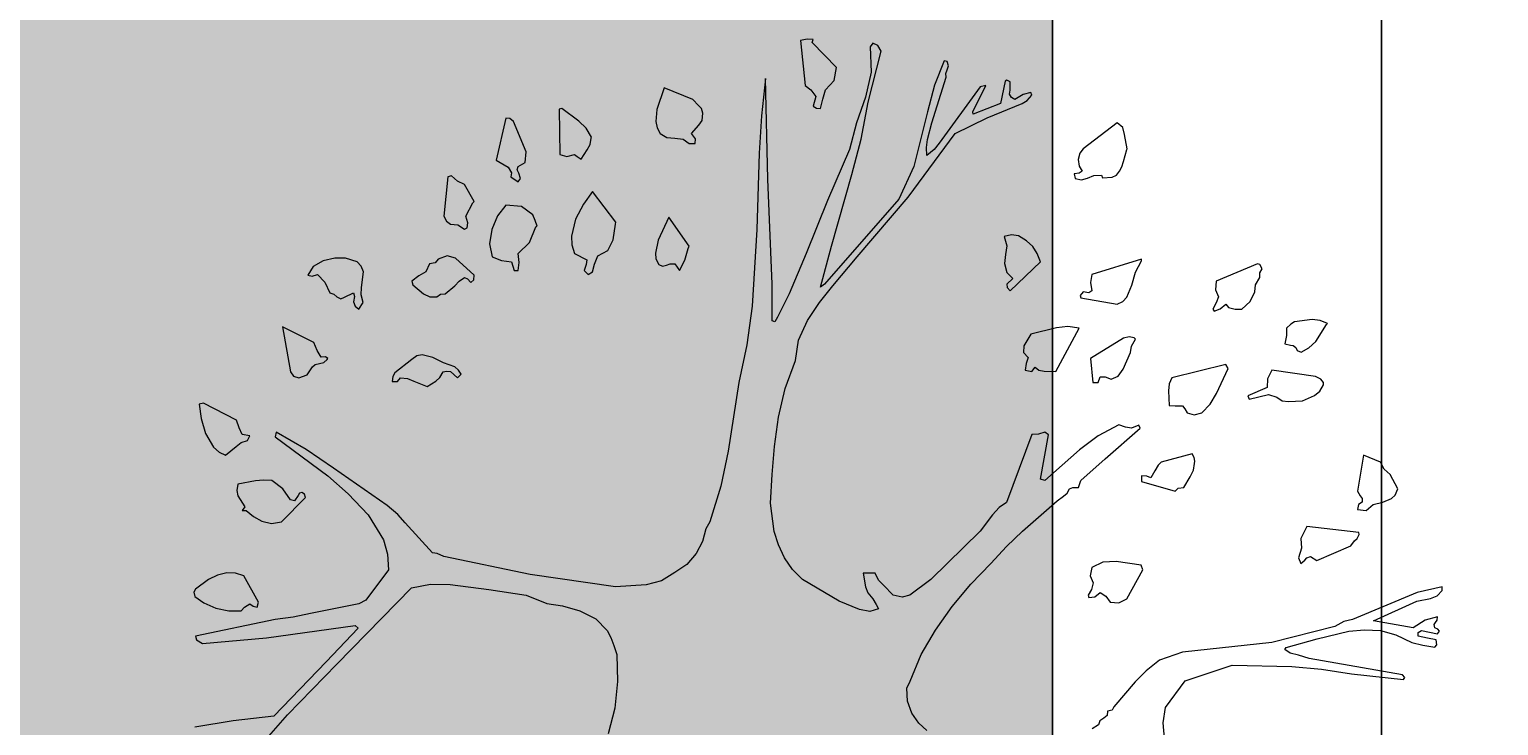
# Model space of a CAD drawing. Units: inches. Extents: x 84 to 1044, y -280 to 906.
# Tile 44 of 105: x 955 to 995, y -107 to -88. Entities that reach past the tile are written whole.
import ezdxf

# ---------------------------------------------------------------- set-up
doc = ezdxf.new("R2010")
doc.units = ezdxf.units.IN
for name, color, linetype, lineweight in [('A-ANNO-DIMS', 2, 'Continuous', 18), ('C-PROP', 7, 'Continuous', 25), ('L-PLNT', 114, 'Continuous', 15)]:
    doc.layers.add(name, color=color, linetype=linetype, lineweight=lineweight)
doc.layers.add('L-PLNT-PATT', color=9, linetype='Continuous', lineweight=9, true_color=0xafd9aa)
doc.styles.get("Standard").update_dxf_attribs({"font": 'arial.ttf'})
doc.dimstyles.get("Standard").update_dxf_attribs({"dimtxt": 0.18, "dimasz": 0.18, "dimexe": 0.18, "dimexo": 0.0625, "dimgap": 0.09, "dimtad": 0, "dimtih": 1, "dimtoh": 1, "dimdec": 4, "dimzin": 0, "dimdsep": 46, "dimtxsty": 'Standard', "dimcen": 0.09, "dimadec": 0, "dimazin": 0, "dimtfac": 1, "dimtdec": 4, "dimtofl": 0, "dimtmove": 0, "dimatfit": 3, "dimfxl": 1, "dimtolj": 1, "dimtzin": 0, "dimarcsym": 0})

# ---------------------------------------------------------------- blocks, each defined once
blk = doc.blocks.new('A$C37E508DF')
for p, q in [((0.6329, 1.5111), (0.6367, 1.5175)), ((0.6367, 1.5175), (0.6423, 1.5201)), ((0.6423, 1.5201), (0.6453, 1.5158)), ((0.6826, 1.493), (0.7096, 1.5209)), ((0.7083, 1.5239), (0.7152, 1.5244)), ((0.7096, 1.5209), (0.7083, 1.5239)), ((0.7152, 1.5244), (0.7225, 1.5231)), ((0.7225, 1.5231), (0.7174, 1.4729)), ((0.5596, 1.4995), (0.563, 1.5003)), ((0.563, 1.5003), (0.5737, 1.4733)), ((0.6475, 1.4545), (0.6329, 1.5111)), ((0.6453, 1.5158), (0.644, 1.4879)), ((0.5583, 1.4948), (0.5596, 1.4995)), ((0.5596, 1.4905), (0.5583, 1.4948)), ((0.5613, 1.4862), (0.5596, 1.4905)), ((0.5608, 1.4823), (0.5613, 1.4862)), ((0.644, 1.4879), (0.6505, 1.46)), ((0.6852, 1.4785), (0.6826, 1.493)), ((0.4897, 1.4772), (0.4935, 1.4789)), ((0.4897, 1.4678), (0.4897, 1.4772)), ((0.4905, 1.4635), (0.4897, 1.4678)), ((0.4935, 1.4789), (0.4952, 1.478)), ((0.4952, 1.478), (0.5004, 1.4532)), ((0.5313, 1.4437), (0.5167, 1.4729)), ((0.5167, 1.4729), (0.5231, 1.4716)), ((0.5231, 1.4716), (0.5686, 1.409)), ((0.5767, 1.4317), (0.5608, 1.4823)), ((0.5737, 1.4733), (0.5814, 1.4437)), ((0.6946, 1.4682), (0.6852, 1.4785)), ((0.6976, 1.4579), (0.6946, 1.4682)), ((0.7109, 1.4682), (0.7053, 1.4609)), ((0.7174, 1.4729), (0.7109, 1.4682)), ((0.7589, 1.3691), (0.7615, 1.481)), ((0.7615, 1.481), (0.7658, 1.4395)), ((0.8421, 1.4575), (0.8739, 1.4703)), ((0.8739, 1.4703), (0.882, 1.4463)), ((0.4657, 1.4622), (0.4669, 1.4652)), ((0.4708, 1.4566), (0.4657, 1.4622)), ((0.4669, 1.4652), (0.4755, 1.463)), ((0.4764, 1.4532), (0.4708, 1.4566)), ((0.4755, 1.463), (0.4845, 1.4575)), ((0.5154, 1.4373), (0.4764, 1.4532)), ((0.4845, 1.4575), (0.4884, 1.4596)), ((0.4884, 1.4596), (0.4905, 1.4635)), ((0.5004, 1.4532), (0.5308, 1.4412)), ((0.6552, 1.4137), (0.6475, 1.4545)), ((0.6505, 1.46), (0.6603, 1.4317)), ((0.7002, 1.4476), (0.6976, 1.4579)), ((0.7053, 1.4609), (0.7083, 1.4502)), ((0.8357, 1.451), (0.8421, 1.4575)), ((0.551, 1.4197), (0.5154, 1.4373)), ((0.5308, 1.4412), (0.5313, 1.4437)), ((0.5814, 1.4437), (0.5969, 1.3833)), ((0.7049, 1.448), (0.7002, 1.4476)), ((0.7083, 1.4502), (0.7049, 1.448)), ((0.7658, 1.4395), (0.7684, 1.3979)), ((0.831, 1.4424), (0.8323, 1.4476)), ((0.8318, 1.4343), (0.831, 1.4424)), ((0.8323, 1.4476), (0.8357, 1.451)), ((0.882, 1.4463), (0.8829, 1.433)), ((0.9686, 1.4334), (0.9875, 1.4476)), ((0.9875, 1.4476), (0.9905, 1.4467)), ((0.9905, 1.4467), (0.9896, 1.3966)), ((1.0411, 1.433), (1.045, 1.4365)), ((1.045, 1.4365), (1.0497, 1.4369)), ((1.0497, 1.4369), (1.0604, 1.3901)), ((0.3598, 1.403), (0.3628, 1.4189)), ((0.3628, 1.4189), (0.3649, 1.4266)), ((0.3649, 1.4266), (0.3709, 1.4317)), ((0.3709, 1.4317), (0.4086, 1.403)), ((0.6029, 1.3494), (0.551, 1.4197)), ((0.5814, 1.4133), (0.5767, 1.4317)), ((0.6603, 1.4317), (0.668, 1.4021)), ((0.8353, 1.4292), (0.8318, 1.4343)), ((0.8434, 1.4197), (0.8353, 1.4292)), ((0.8391, 1.4141), (0.8434, 1.4197)), ((0.8781, 1.4197), (0.8709, 1.4154)), ((0.8816, 1.4262), (0.8781, 1.4197)), ((0.8829, 1.433), (0.8816, 1.4262)), ((0.9545, 1.4159), (0.9605, 1.4257)), ((0.9605, 1.4257), (0.9686, 1.4334)), ((1.0269, 1.3996), (1.0411, 1.433)), ((0.3602, 1.4021), (0.3598, 1.403)), ((0.4086, 1.403), (0.4125, 1.3979)), ((0.5686, 1.409), (0.5741, 1.4021)), ((0.5827, 1.4043), (0.5814, 1.4133)), ((0.5823, 1.3953), (0.5827, 1.4043)), ((0.6655, 1.3743), (0.6552, 1.4137)), ((0.8395, 1.4086), (0.8391, 1.4141)), ((0.846, 1.4086), (0.8395, 1.4086)), ((0.8528, 1.4137), (0.846, 1.4086)), ((0.8619, 1.4146), (0.8528, 1.4137)), ((0.8709, 1.4154), (0.8619, 1.4146)), ((0.9549, 1.4146), (0.9545, 1.4159)), ((0.9558, 1.4077), (0.9549, 1.4146)), ((0.9592, 1.4017), (0.9558, 1.4077)), ((0.364, 1.3888), (0.3602, 1.4021)), ((0.3657, 1.3828), (0.364, 1.3888)), ((0.4125, 1.3979), (0.4142, 1.391)), ((0.4142, 1.391), (0.4134, 1.3837)), ((0.5741, 1.4021), (0.5823, 1.3953)), ((0.668, 1.4021), (0.6925, 1.3455)), ((0.7684, 1.3979), (0.771, 1.3134)), ((0.966, 1.3914), (0.9592, 1.4017)), ((0.9703, 1.3944), (0.966, 1.3914)), ((0.9733, 1.3966), (0.9703, 1.3944)), ((0.9819, 1.3944), (0.9733, 1.3966)), ((0.9896, 1.3966), (0.9819, 1.3944)), ((1.0282, 1.3876), (1.0269, 1.3996)), ((1.0359, 1.3833), (1.0282, 1.3876)), ((1.0604, 1.3901), (1.0471, 1.3824)), ((0.3683, 1.3781), (0.3657, 1.3828)), ((0.3718, 1.3738), (0.3683, 1.3781)), ((0.3765, 1.3713), (0.3718, 1.3738)), ((0.3872, 1.3708), (0.3765, 1.3713)), ((0.3885, 1.3738), (0.3872, 1.3708)), ((0.3971, 1.3734), (0.3885, 1.3738)), ((0.4039, 1.3704), (0.3971, 1.3734)), ((0.4108, 1.3683), (0.4039, 1.3704)), ((0.4134, 1.3837), (0.4099, 1.3781)), ((0.4099, 1.3781), (0.4134, 1.376)), ((0.4176, 1.37), (0.4108, 1.3683)), ((0.4134, 1.376), (0.4189, 1.3751)), ((0.4189, 1.3751), (0.4176, 1.37)), ((0.5969, 1.3833), (0.6132, 1.3472)), ((0.6882, 1.2949), (0.6655, 1.3743)), ((1.0334, 1.37), (1.0351, 1.376)), ((1.0359, 1.3661), (1.0334, 1.37)), ((1.0351, 1.376), (1.0368, 1.3794)), ((1.0368, 1.3794), (1.0359, 1.3833)), ((1.0441, 1.3717), (1.0359, 1.3661)), ((1.0471, 1.3824), (1.0432, 1.3764)), ((1.0432, 1.3764), (1.0441, 1.3717)), ((1.1033, 1.367), (1.1097, 1.373)), ((1.1097, 1.373), (1.114, 1.3717)), ((1.114, 1.3717), (1.1183, 1.328)), ((0.7538, 1.2529), (0.7589, 1.3691)), ((0.9274, 1.3215), (0.9532, 1.3554)), ((0.9532, 1.3554), (0.9635, 1.3413)), ((1.0848, 1.3443), (1.0955, 1.3631)), ((1.0955, 1.3631), (1.1033, 1.367)), ((0.6595, 1.2829), (0.6029, 1.3494)), ((0.6132, 1.3472), (0.6959, 1.2529)), ((0.6925, 1.3455), (0.7161, 1.2868)), ((0.9635, 1.3413), (0.9721, 1.325)), ((1.0197, 1.3297), (1.0321, 1.3387)), ((1.0321, 1.3387), (1.0497, 1.3404)), ((1.0497, 1.3404), (1.0587, 1.3284)), ((1.0861, 1.343), (1.0848, 1.3443)), ((1.0938, 1.328), (1.0861, 1.343)), ((0.846, 1.2949), (0.8687, 1.3271)), ((0.8687, 1.3271), (0.8803, 1.3014)), ((0.9279, 1.3194), (0.9274, 1.3215)), ((0.9721, 1.325), (0.9768, 1.3061)), ((1.0149, 1.3172), (1.0171, 1.3232)), ((1.0171, 1.3232), (1.0197, 1.3297)), ((1.0587, 1.3284), (1.0651, 1.3134)), ((1.0917, 1.3207), (1.0938, 1.328)), ((1.1153, 1.3228), (1.111, 1.3194)), ((1.1183, 1.328), (1.1153, 1.3228)), ((0.4717, 1.3009), (0.4807, 1.3065)), ((0.4807, 1.3065), (0.4884, 1.3074)), ((0.4884, 1.3074), (0.4965, 1.3057)), ((0.4965, 1.3057), (0.4935, 1.2954)), ((0.771, 1.3134), (0.7761, 1.2285)), ((0.9305, 1.3018), (0.9279, 1.3194)), ((0.9768, 1.3061), (0.9763, 1.2962)), ((1.0162, 1.3164), (1.0149, 1.3172)), ((1.0231, 1.2988), (1.0162, 1.3164)), ((1.0651, 1.3134), (1.0677, 1.2975)), ((1.0925, 1.3151), (1.0917, 1.3207)), ((1.0955, 1.3138), (1.0925, 1.3151)), ((1.1028, 1.3185), (1.0955, 1.3138)), ((1.111, 1.3194), (1.1028, 1.3185)), ((0.4597, 1.2868), (0.4648, 1.2945)), ((0.4648, 1.2945), (0.4717, 1.3009)), ((0.4935, 1.2954), (0.4948, 1.2855)), ((0.7002, 1.2495), (0.6882, 1.2949)), ((0.8473, 1.2924), (0.846, 1.2949)), ((0.8507, 1.2795), (0.8473, 1.2924)), ((0.8803, 1.3014), (0.8833, 1.2872)), ((0.9365, 1.2902), (0.9305, 1.3018)), ((0.9476, 1.2842), (0.9365, 1.2902)), ((0.9763, 1.2962), (0.9733, 1.2868)), ((1.0359, 1.2868), (1.0231, 1.2988)), ((1.0677, 1.2975), (1.0647, 1.2829)), ((0.2101, 1.2696), (0.2127, 1.2744)), ((0.2127, 1.2744), (0.2152, 1.2752)), ((0.2152, 1.2752), (0.2611, 1.2559)), ((0.3439, 1.2804), (0.3992, 1.2636)), ((0.3439, 1.2787), (0.3439, 1.2804)), ((0.3507, 1.2662), (0.3439, 1.2787)), ((0.4562, 1.2774), (0.4597, 1.2868)), ((0.4897, 1.2452), (0.4562, 1.2774)), ((0.4961, 1.2756), (0.4935, 1.2658)), ((0.4948, 1.2855), (0.4961, 1.2756)), ((0.6865, 1.2508), (0.6595, 1.2829)), ((0.7161, 1.2868), (0.7349, 1.2422)), ((0.8567, 1.2679), (0.8507, 1.2795)), ((0.8619, 1.2752), (0.8567, 1.2679)), ((0.867, 1.2752), (0.8619, 1.2752)), ((0.8713, 1.2739), (0.867, 1.2752)), ((0.8756, 1.2726), (0.8713, 1.2739)), ((0.8799, 1.2744), (0.8756, 1.2726)), ((0.8829, 1.2808), (0.8799, 1.2744)), ((0.8833, 1.2872), (0.8829, 1.2808)), ((0.951, 1.2748), (0.9476, 1.2842)), ((0.9532, 1.2666), (0.951, 1.2748)), ((0.9733, 1.2868), (0.9596, 1.2799)), ((0.9596, 1.2799), (0.9605, 1.2744)), ((0.9605, 1.2744), (0.9626, 1.2679)), ((1.0347, 1.2769), (1.0359, 1.2868)), ((1.0359, 1.2679), (1.0347, 1.2769)), ((1.0432, 1.2774), (1.0402, 1.2679)), ((1.0544, 1.2791), (1.0432, 1.2774)), ((1.0647, 1.2829), (1.0544, 1.2791)), ((1.0848, 1.2628), (1.1054, 1.2817)), ((1.1054, 1.2817), (1.1148, 1.2842)), ((1.1148, 1.2842), (1.1247, 1.2804)), ((1.1247, 1.2804), (1.1281, 1.2765)), ((1.1281, 1.2765), (1.1341, 1.2752)), ((1.1341, 1.2752), (1.1384, 1.2666)), ((1.2075, 1.2666), (1.21, 1.2726)), ((1.21, 1.2726), (1.2147, 1.2774)), ((1.2147, 1.2774), (1.2276, 1.2817)), ((1.2276, 1.2817), (1.2392, 1.2817)), ((1.2392, 1.2817), (1.2521, 1.2787)), ((1.2521, 1.2787), (1.2632, 1.2722)), ((1.2632, 1.2722), (1.2692, 1.2628)), ((0.2127, 1.2654), (0.2101, 1.2696)), ((0.2127, 1.2602), (0.2127, 1.2654)), ((0.2174, 1.2521), (0.2127, 1.2602)), ((0.2611, 1.2559), (0.262, 1.2465)), ((0.3546, 1.2516), (0.3507, 1.2662)), ((0.3992, 1.2636), (0.4005, 1.2546)), ((0.4935, 1.2658), (0.4867, 1.2589)), ((0.4867, 1.2589), (0.4935, 1.2529)), ((0.9583, 1.2636), (0.9532, 1.2666)), ((0.9626, 1.2679), (0.9583, 1.2636)), ((1.0402, 1.2679), (1.0359, 1.2679)), ((1.0852, 1.2576), (1.0848, 1.2628)), ((1.0883, 1.2546), (1.0852, 1.2576)), ((1.0921, 1.2585), (1.0883, 1.2546)), ((1.0955, 1.2602), (1.0921, 1.2585)), ((1.1015, 1.2559), (1.0955, 1.2602)), ((1.1063, 1.2508), (1.1015, 1.2559)), ((1.1384, 1.2666), (1.1461, 1.2619)), ((1.1461, 1.2619), (1.1539, 1.2559)), ((1.1539, 1.2559), (1.1526, 1.2521)), ((1.2096, 1.2491), (1.2075, 1.2666)), ((1.2585, 1.2636), (1.2503, 1.2551)), ((1.2645, 1.2615), (1.2585, 1.2636)), ((1.2692, 1.2628), (1.2645, 1.2615)), ((0.2182, 1.2443), (0.2174, 1.2521)), ((0.2234, 1.2336), (0.2182, 1.2443)), ((0.262, 1.2465), (0.2586, 1.2388)), ((0.3602, 1.2383), (0.3546, 1.2516)), ((0.4005, 1.2546), (0.3992, 1.2452)), ((0.3992, 1.2452), (0.4026, 1.2431)), ((0.4026, 1.2431), (0.4086, 1.2443)), ((0.4086, 1.2443), (0.4121, 1.2401)), ((0.4121, 1.2401), (0.4112, 1.2375)), ((0.4931, 1.2491), (0.4897, 1.2452)), ((0.4935, 1.2529), (0.4931, 1.2491)), ((0.7015, 1.2323), (0.6865, 1.2508)), ((0.6959, 1.2529), (0.7002, 1.2495)), ((0.7349, 1.2422), (0.7482, 1.216)), ((0.7538, 1.2122), (0.7538, 1.2529)), ((1.117, 1.2422), (1.1063, 1.2508)), ((1.1221, 1.2418), (1.117, 1.2422)), ((1.126, 1.2388), (1.1221, 1.2418)), ((1.141, 1.2422), (1.1337, 1.2388)), ((1.1526, 1.2521), (1.141, 1.2422)), ((1.2079, 1.2323), (1.21, 1.2409)), ((1.21, 1.2409), (1.2096, 1.2491)), ((1.2186, 1.2431), (1.2173, 1.2392)), ((1.2285, 1.2383), (1.2186, 1.2431)), ((1.2405, 1.2418), (1.2371, 1.2388)), ((1.2448, 1.2431), (1.2405, 1.2418)), ((1.2503, 1.2551), (1.2448, 1.2431)), ((0.2328, 1.2251), (0.2234, 1.2336)), ((0.2401, 1.2251), (0.2328, 1.2251)), ((0.2474, 1.2268), (0.2401, 1.2251)), ((0.2504, 1.2306), (0.2474, 1.2268)), ((0.2568, 1.2255), (0.2504, 1.2306)), ((0.2633, 1.2229), (0.2568, 1.2255)), ((0.2586, 1.2388), (0.2611, 1.2319)), ((0.2611, 1.2319), (0.265, 1.2251)), ((0.265, 1.2251), (0.2633, 1.2229)), ((0.3649, 1.2336), (0.3602, 1.2383)), ((0.3709, 1.2306), (0.3649, 1.2336)), ((0.4112, 1.2375), (0.3709, 1.2306)), ((0.7148, 1.2126), (0.7015, 1.2323)), ((0.7761, 1.2285), (0.7821, 1.1856)), ((1.1337, 1.2388), (1.126, 1.2388)), ((1.2126, 1.2251), (1.2079, 1.2323)), ((1.2169, 1.2285), (1.2126, 1.2251)), ((1.2186, 1.2332), (1.2169, 1.2285)), ((1.2173, 1.2392), (1.2186, 1.2332)), ((1.2328, 1.2366), (1.2285, 1.2383)), ((1.2371, 1.2388), (1.2328, 1.2366)), ((0.1376, 1.2092), (0.1458, 1.2126)), ((0.1389, 1.2079), (0.1376, 1.2092)), ((0.1505, 1.189), (0.1389, 1.2079)), ((0.1458, 1.2126), (0.1548, 1.2135)), ((0.1548, 1.2135), (0.1741, 1.2109)), ((0.1741, 1.2109), (0.1784, 1.2083)), ((0.1784, 1.2083), (0.1831, 1.204)), ((0.7246, 1.1908), (0.7148, 1.2126)), ((0.7482, 1.216), (0.7508, 1.2109)), ((0.7508, 1.2109), (0.7538, 1.2122)), ((0.1831, 1.204), (0.1831, 1.1959)), ((0.1831, 1.1959), (0.1848, 1.1865)), ((0.3507, 1.1916), (0.352, 1.1933)), ((0.355, 1.1839), (0.3507, 1.1916)), ((0.352, 1.1933), (0.3576, 1.1942)), ((0.3576, 1.1942), (0.364, 1.1929)), ((0.364, 1.1929), (0.4005, 1.1702)), ((0.4134, 1.204), (0.4258, 1.2058)), ((0.4391, 1.156), (0.4134, 1.204)), ((0.4258, 1.2058), (0.4382, 1.2045)), ((0.4382, 1.2045), (0.4669, 1.1972)), ((0.4669, 1.1972), (0.4747, 1.1843)), ((0.7281, 1.168), (0.7246, 1.1908)), ((1.2628, 1.1882), (1.2975, 1.2053)), ((1.2975, 1.2053), (1.2885, 1.1556)), ((0.1582, 1.1822), (0.1505, 1.189)), ((0.1668, 1.1775), (0.1582, 1.1822)), ((0.1711, 1.1792), (0.1668, 1.1775)), ((0.1728, 1.1826), (0.1711, 1.1792)), ((0.1758, 1.1847), (0.1728, 1.1826)), ((0.1788, 1.1852), (0.1758, 1.1847)), ((0.1848, 1.1865), (0.1788, 1.1852)), ((0.3563, 1.177), (0.355, 1.1839)), ((0.3645, 1.1586), (0.3563, 1.177)), ((0.4751, 1.177), (0.47, 1.1714)), ((0.4747, 1.1843), (0.4751, 1.177)), ((0.7821, 1.1856), (0.7911, 1.1436)), ((1.1307, 1.1714), (1.1423, 1.1744)), ((1.1423, 1.1744), (1.1483, 1.1732)), ((1.2546, 1.1719), (1.2589, 1.1792)), ((1.2589, 1.1792), (1.2628, 1.1882)), ((0.2478, 1.1594), (0.2504, 1.1637)), ((0.2607, 1.1316), (0.2478, 1.1594)), ((0.2504, 1.1637), (0.3104, 1.1487)), ((0.37, 1.1509), (0.3645, 1.1586)), ((0.4005, 1.1702), (0.3979, 1.1436)), ((0.4622, 1.1607), (0.458, 1.1573)), ((0.4657, 1.156), (0.4622, 1.1607)), ((0.47, 1.1714), (0.4721, 1.1646)), ((0.4721, 1.1646), (0.473, 1.1573)), ((0.7396, 1.1371), (0.7281, 1.168)), ((1.102, 1.1573), (1.1063, 1.1612)), ((1.1063, 1.1612), (1.1187, 1.1655)), ((1.1187, 1.1655), (1.1307, 1.1714)), ((1.1483, 1.1732), (1.1539, 1.1693)), ((1.1539, 1.1693), (1.1727, 1.1543)), ((1.2469, 1.1702), (1.2495, 1.1723)), ((1.2478, 1.1693), (1.2469, 1.1702)), ((1.2516, 1.1659), (1.2478, 1.1693)), ((1.2495, 1.1723), (1.2546, 1.1719)), ((1.2563, 1.1646), (1.2516, 1.1659)), ((1.2611, 1.1637), (1.2563, 1.1646)), ((1.2641, 1.1612), (1.2611, 1.1637)), ((1.2701, 1.1522), (1.2641, 1.1612)), ((0.1419, 1.1436), (0.1449, 1.1474)), ((0.1419, 1.141), (0.1419, 1.1436)), ((0.1449, 1.1474), (0.1509, 1.1504)), ((0.1509, 1.1504), (0.1994, 1.1573)), ((0.1994, 1.1573), (0.2041, 1.1479)), ((0.2041, 1.1479), (0.2045, 1.138)), ((0.3104, 1.1487), (0.3134, 1.1423)), ((0.3134, 1.1423), (0.3139, 1.1346)), ((0.3778, 1.1474), (0.37, 1.1509)), ((0.3842, 1.15), (0.3778, 1.1474)), ((0.3898, 1.15), (0.3842, 1.15)), ((0.3923, 1.1436), (0.3898, 1.15)), ((0.3979, 1.1436), (0.3923, 1.1436)), ((0.4519, 1.1564), (0.4391, 1.156)), ((0.458, 1.1573), (0.4519, 1.1564)), ((0.473, 1.1573), (0.4657, 1.156)), ((0.7911, 1.1436), (0.8027, 1.0677)), ((1.099, 1.153), (1.102, 1.1573)), ((1.1033, 1.1487), (1.099, 1.153)), ((1.111, 1.156), (1.1033, 1.1487)), ((1.1153, 1.1564), (1.111, 1.156)), ((1.1191, 1.1556), (1.1153, 1.1564)), ((1.1226, 1.1492), (1.1191, 1.1556)), ((1.1273, 1.1453), (1.1226, 1.1492)), ((1.1367, 1.1393), (1.1273, 1.1453)), ((1.1517, 1.1453), (1.1367, 1.1393)), ((1.1586, 1.1483), (1.1517, 1.1453)), ((1.1663, 1.1487), (1.1586, 1.1483)), ((1.1697, 1.1449), (1.1663, 1.1487)), ((1.1757, 1.1449), (1.1697, 1.1449)), ((1.1727, 1.1543), (1.1749, 1.1504)), ((1.1749, 1.1504), (1.1757, 1.1449)), ((1.2791, 1.1487), (1.2701, 1.1522)), ((1.2851, 1.1509), (1.2791, 1.1487)), ((1.2885, 1.1556), (1.2851, 1.1509)), ((0.1462, 1.1342), (0.1419, 1.141)), ((0.1522, 1.1294), (0.1462, 1.1342)), ((0.1655, 1.1234), (0.1522, 1.1294)), ((0.1938, 1.1273), (0.1878, 1.1234)), ((0.2032, 1.1303), (0.1938, 1.1273)), ((0.2247, 1.1251), (0.2032, 1.1303)), ((0.2045, 1.138), (0.226, 1.129)), ((0.226, 1.129), (0.2247, 1.1251)), ((0.268, 1.1196), (0.2607, 1.1316)), ((0.3139, 1.1346), (0.3134, 1.1183)), ((0.7469, 1.1054), (0.7396, 1.1371)), ((0.181, 1.1226), (0.1655, 1.1234)), ((0.1878, 1.1234), (0.181, 1.1226)), ((0.277, 1.1101), (0.268, 1.1196)), ((0.2856, 1.108), (0.277, 1.1101)), ((0.2933, 1.1101), (0.2856, 1.108)), ((0.2959, 1.1144), (0.2933, 1.1101)), ((0.2984, 1.1179), (0.2959, 1.1144)), ((0.3066, 1.1179), (0.2984, 1.1179)), ((0.3134, 1.1183), (0.3066, 1.1179)), ((1.3485, 1.102), (1.385, 1.1209)), ((1.385, 1.1209), (1.3897, 1.1196)), ((1.3897, 1.1196), (1.3875, 1.1037)), ((0.3456, 1.093), (0.3469, 1.0964)), ((0.3842, 1.0591), (0.3456, 1.093)), ((0.3469, 1.0964), (0.355, 1.093)), ((0.355, 1.093), (0.3619, 1.0943)), ((0.3619, 1.0943), (0.3692, 1.0968)), ((0.3692, 1.0968), (0.3923, 1.0844)), ((0.7512, 1.0728), (0.7469, 1.1054)), ((1.3421, 1.0861), (1.3455, 1.0934)), ((1.3455, 1.0934), (1.3485, 1.102)), ((1.3875, 1.1037), (1.3828, 1.087)), ((0.3923, 1.0844), (0.4129, 1.069)), ((0.4472, 1.0857), (0.4515, 1.0887)), ((0.4562, 1.0364), (0.4472, 1.0857)), ((0.4515, 1.0887), (0.4584, 1.0865)), ((0.4584, 1.0865), (0.4657, 1.0861)), ((0.4657, 1.0861), (0.4939, 1.0107)), ((1.3057, 1.0835), (1.2469, 1.0402)), ((1.2713, 1.0694), (1.3044, 1.0887)), ((1.3044, 1.0887), (1.3057, 1.0835)), ((1.3335, 1.0844), (1.3421, 1.0861)), ((1.3361, 1.0793), (1.3335, 1.0844)), ((1.3434, 1.0771), (1.3361, 1.0793)), ((1.349, 1.0728), (1.3434, 1.0771)), ((1.3828, 1.087), (1.3738, 1.072)), ((0.0789, 1.0552), (0.0978, 1.063)), ((0.0978, 1.063), (0.1042, 1.0231)), ((0.2847, 1.0565), (0.2856, 1.0604)), ((0.2856, 1.0604), (0.2877, 1.0647)), ((0.2877, 1.0647), (0.3224, 1.0552)), ((0.4129, 1.069), (0.4515, 1.0351)), ((0.7538, 1.0415), (0.7512, 1.0728)), ((0.8027, 1.0677), (0.8108, 1.0287)), ((1.2409, 1.0488), (1.2713, 1.0694)), ((1.3605, 1.063), (1.349, 1.0728)), ((1.3678, 1.0664), (1.3605, 1.063)), ((1.3738, 1.072), (1.3678, 1.0664)), ((0.0682, 1.0415), (0.0746, 1.0475)), ((0.0746, 1.0475), (0.0789, 1.0552)), ((0.2851, 1.054), (0.2847, 1.0565)), ((0.2864, 1.0463), (0.2851, 1.054)), ((0.2899, 1.039), (0.2864, 1.0463)), ((0.3224, 1.0552), (0.3255, 1.0522)), ((0.3255, 1.0522), (0.3293, 1.0458)), ((0.3293, 1.0458), (0.3336, 1.0381)), ((0.4112, 1.0351), (0.3842, 1.0591)), ((1.1813, 1.0072), (1.2409, 1.0488)), ((0.0596, 1.0257), (0.0682, 1.0415)), ((0.2972, 1.0274), (0.2899, 1.039)), ((0.3032, 1.0265), (0.2972, 1.0274)), ((0.3439, 1.0338), (0.3066, 1.0231)), ((0.3336, 1.0381), (0.3383, 1.0398)), ((0.3383, 1.0398), (0.3439, 1.0402)), ((0.3439, 1.0402), (0.3439, 1.0338)), ((0.4138, 1.0274), (0.4112, 1.0351)), ((0.4202, 1.0274), (0.4138, 1.0274)), ((0.4241, 1.0257), (0.4202, 1.0274)), ((0.4515, 1.0351), (0.4562, 1.0364)), ((0.7559, 1.0098), (0.7538, 1.0415)), ((0.8108, 1.0287), (0.8233, 0.9892)), ((1.2469, 1.0402), (1.2246, 1.0201)), ((1.2971, 1.0257), (1.3091, 1.0351)), ((1.3091, 1.0351), (1.3185, 1.0355)), ((1.3185, 1.0355), (1.3275, 1.0347)), ((1.3275, 1.0347), (1.3468, 1.0308)), ((1.3468, 1.0308), (1.3481, 1.0239)), ((0.0626, 1.0188), (0.0596, 1.0257)), ((0.0665, 1.0149), (0.0626, 1.0188)), ((0.0763, 1.0111), (0.0665, 1.0149)), ((0.087, 1.0085), (0.0763, 1.0111)), ((0.1012, 1.018), (0.099, 1.0149)), ((0.099, 1.0149), (0.099, 1.0111)), ((0.099, 1.0111), (0.1033, 1.0085)), ((0.1042, 1.0231), (0.1012, 1.018)), ((0.3066, 1.0231), (0.3032, 1.0265)), ((0.4267, 1.0209), (0.4241, 1.0257)), ((0.4305, 1.0175), (0.4267, 1.0209)), ((0.4378, 1.0124), (0.4305, 1.0175)), ((0.476, 0.9789), (0.4378, 1.0124)), ((1.2246, 1.0201), (1.2023, 0.9969)), ((1.2718, 1.0162), (1.2731, 1.0197)), ((1.2984, 0.9892), (1.2718, 1.0162)), ((1.2731, 1.0197), (1.2761, 1.0218)), ((1.2761, 1.0218), (1.2786, 1.0209)), ((1.2786, 1.0209), (1.2799, 1.0184)), ((1.2799, 1.0184), (1.2842, 1.0124)), ((1.2842, 1.0124), (1.2885, 1.0136)), ((1.2885, 1.0136), (1.2971, 1.0257)), ((1.3468, 1.018), (1.3391, 1.0059)), ((1.3481, 1.0239), (1.3468, 1.018)), ((0.0948, 1.0016), (0.087, 1.0085)), ((0.1042, 1.0029), (0.0948, 1.0016)), ((0.1033, 1.0085), (0.1042, 1.0029)), ((0.4939, 1.0107), (0.5021, 1.0051)), ((0.5021, 1.0051), (0.5094, 0.9969)), ((0.5094, 0.9969), (0.5231, 0.9789)), ((0.7516, 0.9785), (0.7559, 1.0098)), ((1.1612, 0.9879), (1.1693, 0.9974)), ((1.1693, 0.9974), (1.1813, 1.0072)), ((1.2023, 0.9969), (1.1852, 0.9691)), ((1.3297, 0.9952), (1.3202, 0.9901)), ((1.3378, 1.0016), (1.3297, 0.9952)), ((1.3421, 1.0016), (1.3378, 1.0016)), ((1.3391, 1.0059), (1.3421, 1.0016)), ((0.1029, 0.9772), (0.1604, 0.9841)), ((0.1604, 0.9841), (0.1672, 0.9708)), ((0.4939, 0.9618), (0.476, 0.9789)), ((0.5231, 0.9789), (0.578, 0.9253)), ((0.7469, 0.9635), (0.7516, 0.9785)), ((0.8233, 0.9892), (0.8275, 0.9815)), ((0.8275, 0.9815), (0.8314, 0.9673)), ((1.1311, 0.9549), (1.1612, 0.9879)), ((1.3095, 0.9875), (1.2984, 0.9892)), ((1.3202, 0.9901), (1.3095, 0.9875)), ((0.1025, 0.9751), (0.1029, 0.9772)), ((0.1046, 0.9708), (0.1025, 0.9751)), ((0.1076, 0.9682), (0.1046, 0.9708)), ((0.1119, 0.9626), (0.1076, 0.9682)), ((0.1496, 0.9463), (0.1119, 0.9626)), ((0.1672, 0.9708), (0.1664, 0.9601)), ((0.7401, 0.9493), (0.7469, 0.9635)), ((0.8314, 0.9673), (0.8383, 0.954)), ((1.1852, 0.9691), (1.1809, 0.9532)), ((0.1565, 0.9506), (0.1496, 0.9463)), ((0.1604, 0.9493), (0.1565, 0.9506)), ((0.1629, 0.9468), (0.1604, 0.9493)), ((0.1672, 0.9429), (0.1629, 0.9468)), ((0.1664, 0.9601), (0.1698, 0.9493)), ((0.1698, 0.9493), (0.1672, 0.9429)), ((0.5111, 0.9429), (0.4939, 0.9618)), ((0.7315, 0.9365), (0.7401, 0.9493)), ((0.8383, 0.954), (0.8486, 0.942)), ((1.0227, 0.9309), (1.1183, 0.9506)), ((1.1183, 0.9506), (1.1256, 0.954)), ((1.1256, 0.954), (1.1311, 0.9549)), ((1.1809, 0.9532), (1.1796, 0.936)), ((0.3426, 0.936), (0.3443, 0.9412)), ((0.3602, 0.9039), (0.3426, 0.936)), ((0.3443, 0.9412), (0.3722, 0.9451)), ((0.3722, 0.9451), (0.3868, 0.9446)), ((0.3868, 0.9446), (0.3992, 0.9386)), ((0.3992, 0.9386), (0.4009, 0.9292)), ((0.5334, 0.9202), (0.5111, 0.9429)), ((0.6359, 0.9245), (0.6397, 0.9322)), ((0.6397, 0.9322), (0.653, 0.9322)), ((0.653, 0.9322), (0.6505, 0.9172)), ((0.7203, 0.9253), (0.7315, 0.9365)), ((0.8486, 0.942), (0.8619, 0.933)), ((0.8619, 0.933), (0.8769, 0.9236)), ((0.9279, 0.9172), (1.0227, 0.9309)), ((1.1796, 0.936), (1.2049, 0.9022)), ((1.3404, 0.9292), (1.3494, 0.9322)), ((1.3494, 0.9322), (1.3592, 0.9326)), ((1.3592, 0.9326), (1.3695, 0.93)), ((1.3695, 0.93), (1.3794, 0.9253)), ((0.0103, 0.9129), (0.0103, 0.9172)), ((0.0103, 0.9172), (0.0382, 0.9107)), ((0.4009, 0.9292), (0.3975, 0.9215)), ((0.3975, 0.9215), (0.3996, 0.9142)), ((0.3996, 0.9142), (0.4031, 0.9077)), ((0.554, 0.8953), (0.5334, 0.9202)), ((0.578, 0.9253), (0.6011, 0.9077)), ((0.6196, 0.9077), (0.6303, 0.9189)), ((0.6303, 0.9189), (0.6359, 0.9245)), ((0.6505, 0.9172), (0.6479, 0.9103)), ((0.6796, 0.9013), (0.7203, 0.9253)), ((0.8769, 0.9236), (0.8936, 0.9193)), ((0.8936, 0.9193), (0.9279, 0.9172)), ((1.0685, 0.9142), (1.0269, 0.9077)), ((1.1114, 0.9198), (1.0685, 0.9142)), ((1.1333, 0.9202), (1.1114, 0.9198)), ((1.1543, 0.9159), (1.1333, 0.9202)), ((1.2371, 0.8314), (1.1543, 0.9159)), ((1.3241, 0.9), (1.3404, 0.9292)), ((1.3794, 0.9253), (1.394, 0.9146)), ((1.394, 0.9146), (1.3957, 0.9112)), ((0.0159, 0.9073), (0.0103, 0.9129)), ((0.0232, 0.9043), (0.0159, 0.9073)), ((0.0386, 0.9013), (0.0232, 0.9043)), ((0.0382, 0.9107), (0.1098, 0.8807)), ((0.0866, 0.8794), (0.0386, 0.9013)), ((0.3692, 0.8992), (0.3602, 0.9039)), ((0.379, 0.9), (0.3692, 0.8992)), ((0.3838, 0.9069), (0.379, 0.9)), ((0.3898, 0.9107), (0.3838, 0.9069)), ((0.3958, 0.906), (0.3898, 0.9107)), ((0.4026, 0.9052), (0.3958, 0.906)), ((0.4031, 0.9077), (0.4026, 0.9052)), ((0.6011, 0.9077), (0.6097, 0.9056)), ((0.6097, 0.9056), (0.6196, 0.9077)), ((0.6384, 0.8974), (0.6359, 0.8927)), ((0.6423, 0.9039), (0.6384, 0.8974)), ((0.6479, 0.9103), (0.6423, 0.9039)), ((0.6569, 0.8919), (0.6796, 0.9013)), ((1.0042, 0.8987), (0.9866, 0.8962)), ((1.0269, 0.9077), (1.0042, 0.8987)), ((1.2049, 0.9022), (1.2126, 0.8983)), ((1.2126, 0.8983), (1.2662, 0.8876)), ((1.3254, 0.8944), (1.3241, 0.9)), ((1.3335, 0.8983), (1.3301, 0.8957)), ((1.3395, 0.8944), (1.3335, 0.8983)), ((1.3846, 0.8992), (1.3713, 0.8936)), ((1.3948, 0.9065), (1.3846, 0.8992)), ((1.3957, 0.9112), (1.3948, 0.9065)), ((0.0159, 0.8803), (0.0154, 0.8837)), ((0.0154, 0.8837), (0.0292, 0.8803)), ((0.1098, 0.8807), (0.1196, 0.8786)), ((0.5728, 0.8691), (0.554, 0.8953)), ((0.6359, 0.8927), (0.6457, 0.8897)), ((0.6457, 0.8897), (0.6569, 0.8919)), ((0.9498, 0.8816), (0.9369, 0.8687)), ((0.9673, 0.8906), (0.9498, 0.8816)), ((0.9866, 0.8962), (0.9673, 0.8906)), ((1.2662, 0.8876), (1.2855, 0.8833)), ((1.2855, 0.8833), (1.3057, 0.8807)), ((1.3057, 0.8807), (1.394, 0.8623)), ((1.3301, 0.8957), (1.3254, 0.8944)), ((1.3434, 0.8906), (1.3395, 0.8944)), ((1.3571, 0.8906), (1.3434, 0.8906)), ((1.3713, 0.8936), (1.3571, 0.8906)), ((0.0133, 0.8679), (0.015, 0.87)), ((0.0154, 0.8649), (0.0133, 0.8679)), ((0.015, 0.87), (0.0184, 0.8717)), ((0.0334, 0.8687), (0.0154, 0.8649)), ((0.0176, 0.8777), (0.0159, 0.8803)), ((0.0193, 0.8752), (0.0176, 0.8777)), ((0.0184, 0.8717), (0.0193, 0.8752)), ((0.0292, 0.8803), (0.0424, 0.8717)), ((0.0369, 0.8666), (0.0334, 0.8687)), ((0.0369, 0.8623), (0.0369, 0.8666)), ((0.0424, 0.8717), (0.0866, 0.8794)), ((0.0789, 0.8687), (0.0617, 0.864)), ((0.0965, 0.8696), (0.0789, 0.8687)), ((0.1141, 0.8679), (0.0965, 0.8696)), ((0.1492, 0.8593), (0.1141, 0.8679)), ((0.1196, 0.8786), (0.1295, 0.873)), ((0.1295, 0.873), (0.1994, 0.8554)), ((0.5887, 0.8421), (0.5728, 0.8691)), ((0.9369, 0.8687), (0.933, 0.861)), ((1.2169, 0.8743), (1.2135, 0.8713)), ((1.2135, 0.8713), (1.2491, 0.834)), ((1.3151, 0.8606), (1.2169, 0.8743)), ((0.0163, 0.8529), (0.0171, 0.8584)), ((0.0184, 0.8503), (0.0163, 0.8529)), ((0.0171, 0.8584), (0.0266, 0.8602)), ((0.0317, 0.8524), (0.0184, 0.8503)), ((0.0266, 0.8602), (0.0369, 0.8623)), ((0.0442, 0.8554), (0.0317, 0.8524)), ((0.0617, 0.864), (0.0442, 0.8554)), ((0.1835, 0.8499), (0.1492, 0.8593)), ((0.1848, 0.8477), (0.1835, 0.8499)), ((0.1994, 0.8554), (0.2984, 0.8447)), ((0.9296, 0.852), (0.9262, 0.8421)), ((0.933, 0.861), (0.9296, 0.852)), ((1.3863, 0.8541), (1.3151, 0.8606)), ((1.3927, 0.8584), (1.3863, 0.8541)), ((1.394, 0.8623), (1.3927, 0.8584)), ((0.0545, 0.8194), (0.1578, 0.8378)), ((0.1578, 0.8378), (0.1698, 0.8413)), ((0.1698, 0.8413), (0.1792, 0.8434)), ((0.1792, 0.8434), (0.1848, 0.8477)), ((0.2984, 0.8447), (0.3242, 0.8357)), ((0.3242, 0.8357), (0.3387, 0.8241)), ((0.6007, 0.8125), (0.5887, 0.8421)), ((0.9262, 0.8421), (0.9257, 0.8121)), ((1.2491, 0.834), (1.3069, 0.7735)), ((0.0519, 0.8164), (0.0545, 0.8194)), ((0.0532, 0.8143), (0.0519, 0.8164)), ((0.1111, 0.8207), (0.0532, 0.8143)), ((0.1441, 0.8258), (0.1111, 0.8207)), ((0.1771, 0.8288), (0.1441, 0.8258)), ((0.2436, 0.8301), (0.1771, 0.8288)), ((0.2954, 0.813), (0.2436, 0.8301)), ((0.3387, 0.8241), (0.3512, 0.8117)), ((1.2919, 0.7752), (1.2371, 0.8314)), ((0.3173, 0.7834), (0.2954, 0.813)), ((0.3512, 0.8117), (0.3748, 0.7842)), ((0.6046, 0.8048), (0.6007, 0.8125)), ((0.6037, 0.7903), (0.6046, 0.8048)), ((0.9257, 0.8121), (0.9287, 0.7825)), ((0.3199, 0.7662), (0.3173, 0.7834)), ((0.3748, 0.7842), (0.3765, 0.7804)), ((0.599, 0.777), (0.6037, 0.7903)), ((0.3765, 0.7804), (0.3816, 0.7791)), ((0.3816, 0.7791), (0.382, 0.7744)), ((0.382, 0.7744), (0.3859, 0.7714)), ((0.3859, 0.7714), (0.3902, 0.7684)), ((0.3902, 0.7684), (0.3919, 0.7641)), ((0.5913, 0.7658), (0.599, 0.777)), ((0.9287, 0.7825), (0.936, 0.7542)), ((1.3151, 0.7487), (1.2919, 0.7752)), ((1.3069, 0.7735), (1.352, 0.7684)), ((1.352, 0.7684), (1.3948, 0.7615)), ((0.3186, 0.7491), (0.3199, 0.7662)), ((0.3919, 0.7641), (0.3988, 0.7598)), ((0.5823, 0.7577), (0.5913, 0.7658))]:
    blk.add_line(p, q)
blk = doc.blocks.new('*D70')
at = {"layer": 'A-ANNO-DIMS', "color": 0, "lineweight": -2, "transparency": 16777216}
for p, q in [((983.136, -64.88), (1043.768, -64.88)), ((1043.588, -65.06), (1043.588, -93.198)), ((1043.588, -121.7), (1043.588, -93.561)), ((992.136, -121.88), (1043.768, -121.88))]:
    blk.add_line(p, q, dxfattribs=at)
at = {"layer": 'A-ANNO-DIMS', "color": 0, "transparency": 16777216}
for points in [[(1043.558, -65.06), (1043.618, -65.06), (1043.588, -64.88)], [(1043.558, -121.7), (1043.618, -121.7), (1043.588, -121.88)]]:
    blk.add_solid(points, dxfattribs=at)
at = {"layer": 'Defpoints', "color": 0, "transparency": 16777216}
for p in [(983.074, -64.88), (1043.588, -64.88), (992.074, -121.88)]:
    blk.add_point(p, dxfattribs=at)
at = {"layer": 'A-ANNO-DIMS', "color": 0, "transparency": 16777216, "insert": (1043.588, -93.38), "char_height": 0.18, "attachment_point": 5}
blk.add_mtext('\\A1;57', dxfattribs=at)

msp = doc.modelspace()

# ---------------------------------------------------------------- hatches: boundary and pattern name
at = {"layer": 'L-PLNT-PATT', "transparency": 33554597}
h = msp.add_hatch(color=256, dxfattribs=at)
h.dxf.hatch_style = 1
h.paths.add_polyline_path([(791.074, 31.12), (791.074, 91.12), (743.074, 91.12), (674.074, 91.12), (674.074, 31.12), (650.074, 31.12), (650.074, -112.88), (983.074, -112.88), (983.074, -64.88), (791.074, -64.88)])

# ---------------------------------------------------------------- linework, layer by layer
at = {"layer": 'C-PROP'}
for points in [[(143.179, -121.88), (134.179, -121.88), (134.179, 856.12), (992.074, 856.12), (992.074, -121.88), (624.574, -121.88)], [(143.179, -112.88), (143.179, 847.12), (983.074, 847.12), (983.074, -112.88), (624.574, -112.88)]]:
    msp.add_lwpolyline(points, dxfattribs=at)

# ---------------------------------------------------------------- block references
at = {"layer": 'L-PLNT', "xscale": -24.64361536662419, "yscale": 24.64361536662419, "zscale": 24.64361536662419}
msp.add_blockref('A$C37E508DF', (993.988, -125.52), dxfattribs=at)

# ---------------------------------------------------------------- dimensions: what is measured, and where the dimension line sits
at = {"layer": 'A-ANNO-DIMS'}
dim = msp.add_linear_dim(base=(1043.588, -64.88), p1=(992.074, -121.88), p2=(983.074, -64.88), angle=90, dimstyle='Standard', override={"dimdec": 0, "dimlfac": 1, "dimrnd": 0, "dimzin": 0, "dimdsep": 46, "dimlunit": 2}, dxfattribs=at)
dim.commit()
dim.dimension.update_dxf_attribs({"geometry": '*D70', "text_midpoint": (1043.588, -93.38)})

doc.saveas('drawing.dxf')
